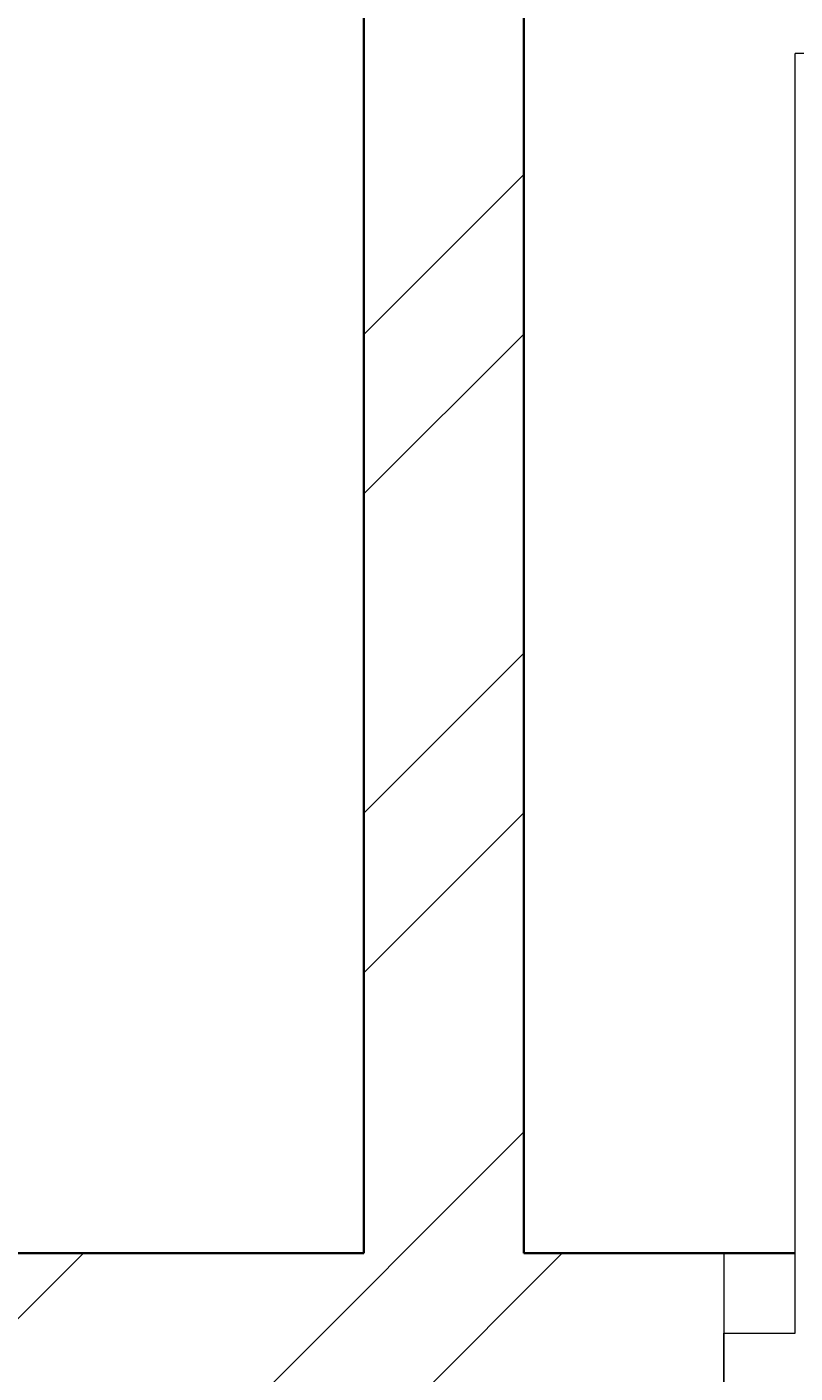
# Model space of a CAD drawing. Units: inches. Extents: x 1962 to 2771, y 1245 to 2660.
# Tile 53 of 114: x 2225 to 2247, y 2030 to 2068. Entities that reach past the tile are written whole.
import ezdxf

# ---------------------------------------------------------------- set-up
doc = ezdxf.new("R2010")
doc.units = ezdxf.units.IN
for name, color, linetype, lineweight in [('A-ANNO-DIMS', 2, 'Continuous', 18), ('A-DOOR', 3, 'Continuous', 18), ('A-WALL', 7, 'Continuous', 35), ('A-WALL-PATT', 252, 'Continuous', 13)]:
    doc.layers.add(name, color=color, linetype=linetype, lineweight=lineweight)
doc.styles.get("Standard").update_dxf_attribs({"font": 'arial.ttf'})
doc.dimstyles.get("Standard").update_dxf_attribs({"dimtxt": 0.18, "dimasz": 0.18, "dimexe": 0.18, "dimexo": 0.0625, "dimgap": 0.09, "dimtad": 0, "dimtih": 1, "dimtoh": 1, "dimdec": 4, "dimzin": 0, "dimdsep": 46, "dimtxsty": 'Standard', "dimcen": 0.09, "dimadec": 0, "dimazin": 0, "dimtfac": 1, "dimtdec": 4, "dimtofl": 0, "dimtmove": 0, "dimatfit": 3, "dimfxl": 1, "dimtolj": 1, "dimtzin": 0, "dimarcsym": 0})

# ---------------------------------------------------------------- blocks, each defined once
blk = doc.blocks.new('*D40')
at = {"layer": 'A-ANNO-DIMS', "color": 0, "lineweight": -2, "transparency": 16777216}
for p, q in [((2072.02, 2033.906), (2072.02, 2583.474)), ((2660.807, 2524.406), (2660.807, 2583.474)), ((2072.2, 2583.294), (2366.02, 2583.294)), ((2660.627, 2583.294), (2366.808, 2583.294))]:
    blk.add_line(p, q, dxfattribs=at)
at = {"layer": 'A-ANNO-DIMS', "color": 0, "transparency": 16777216}
for points in [[(2072.2, 2583.324), (2072.2, 2583.264), (2072.02, 2583.294)], [(2660.627, 2583.324), (2660.627, 2583.264), (2660.807, 2583.294)]]:
    blk.add_solid(points, dxfattribs=at)
at = {"layer": 'Defpoints', "color": 0, "transparency": 16777216}
for p in [(2660.807, 2583.294), (2660.807, 2524.344), (2072.02, 2033.844)]:
    blk.add_point(p, dxfattribs=at)
at = {"layer": 'A-ANNO-DIMS', "color": 0, "transparency": 16777216, "insert": (2366.414, 2583.294), "char_height": 0.18, "attachment_point": 5}
blk.add_mtext('\\A1;588.8', dxfattribs=at)

msp = doc.modelspace()

# ---------------------------------------------------------------- hatches: boundary and pattern name
at = {"layer": 'A-WALL-PATT'}
h = msp.add_hatch(dxfattribs=at)
h.set_pattern_fill('ANSI32', color=256)
h.paths.add_polyline_path([(2090.8074, 2467.3437), (2141.6481, 2467.3437), (2141.6481, 2469.5937), (2141.6481, 2471.8437), (2086.3074, 2471.8437), (2086.3074, 2422.5333), (2090.8074, 2422.5333)])
h.paths.add_polyline_path([(2282.7664, 2471.8437), (2204.8982, 2471.8437), (2204.8982, 2467.3437), (2234.8074, 2467.3437), (2234.8074, 2311.3437), (2228.7492, 2311.3437), (2228.7492, 2306.8437), (2234.8074, 2306.8437), (2331.9227, 2306.8437), (2331.9227, 2309.0937), (2331.9227, 2311.3437), (2239.3074, 2311.3437), (2239.3074, 2467.3437), (2282.7664, 2467.3437), (2282.7664, 2469.5937)])
h.paths.add_polyline_path([(2471.4531, 2519.8437), (2552.011, 2519.8437), (2564.3996, 2519.8437), (2564.3996, 2511.1389), (2568.8996, 2511.1389), (2568.8996, 2524.3437), (2466.9531, 2524.3437), (2466.9531, 2471.8437), (2450.0749, 2471.8437), (2446.4672, 2471.8437), (2446.4672, 2467.3437), (2450.0749, 2467.3437), (2475.9988, 2467.3437), (2475.9988, 2469.5937), (2475.9988, 2471.8437), (2471.4531, 2471.8437)])
h.paths.add_polyline_path([(2575.2231, 2469.5937), (2575.2231, 2471.8437), (2568.8996, 2471.8437), (2568.8996, 2487.1389), (2564.3996, 2487.1389), (2564.3996, 2471.8437), (2556.511, 2471.8437), (2499.2904, 2471.8437), (2499.2904, 2467.3437), (2507.8074, 2467.3437), (2507.8074, 2311.3437), (2414.863, 2311.3437), (2414.863, 2306.8437), (2512.3074, 2306.8437), (2517.0114, 2306.8437), (2517.0114, 2309.0937), (2517.0114, 2311.3437), (2512.3074, 2311.3437), (2512.3074, 2467.3437), (2575.2231, 2467.3437)])
h.paths.add_polyline_path([(2660.8074, 2471.8437), (2600.9602, 2471.8437), (2600.9602, 2467.3437), (2656.3074, 2467.3437), (2656.3074, 2432.5704), (2660.8074, 2432.5704)])
h.paths.add_polyline_path([(2660.8074, 2372.5704), (2656.3074, 2372.5704), (2656.3074, 2311.3437), (2600.276, 2311.3437), (2600.276, 2309.0937), (2600.276, 2306.8437), (2656.3074, 2306.8437), (2656.3074, 2296.2593), (2660.8074, 2296.2593)])
h.paths.add_polyline_path([(2572.3074, 2306.8437), (2577.1385, 2306.8437), (2577.1385, 2311.3437), (2551.082, 2311.3437), (2551.082, 2306.8437), (2567.8074, 2306.8437), (2567.8074, 2258.8437), (2540.0574, 2258.8437), (2540.0574, 2256.5937), (2540.0574, 2254.3437), (2567.8074, 2254.3437), (2656.3074, 2254.3437), (2656.3074, 2236.9085), (2660.8074, 2236.9085), (2660.8074, 2272.2593), (2656.3074, 2272.2593), (2656.3074, 2258.8437), (2572.3074, 2258.8437)])
h.paths.add_polyline_path([(2512.3074, 2254.3437), (2518.8716, 2254.3437), (2518.8716, 2256.5937), (2518.8716, 2258.8437), (2507.8074, 2258.8437), (2507.8074, 2177.8437), (2567.8074, 2177.8437), (2567.8074, 2172.9628), (2572.3074, 2172.9628), (2572.3074, 2177.8437), (2656.3074, 2177.8437), (2656.3074, 2166.4846), (2660.8074, 2166.4846), (2660.8074, 2200.9085), (2656.3074, 2200.9085), (2656.3074, 2182.3437), (2512.3074, 2182.3437)])
h.paths.add_polyline_path([(2656.3074, 2129.8437), (2572.3074, 2129.8437), (2572.3074, 2150.3044), (2570.0574, 2150.3044), (2567.8074, 2150.3044), (2567.8074, 2129.8437), (2507.8074, 2129.8437), (2507.8074, 2116.3027), (2510.0574, 2116.3027), (2512.3074, 2116.3027), (2512.3074, 2125.3437), (2567.8074, 2125.3437), (2572.3074, 2125.3437), (2656.3074, 2125.3437)])
h.paths.add_polyline_path([(2090.8074, 2362.5333), (2086.3074, 2362.5333), (2086.3074, 2298.6242), (2090.8074, 2298.6242), (2090.8074, 2306.8437), (2174.8074, 2306.8437), (2174.8074, 2286.4178), (2179.3074, 2286.4178), (2179.3074, 2306.8437), (2192.8641, 2306.8437), (2192.8641, 2309.0937), (2192.8641, 2311.3437), (2090.8074, 2311.3437)])
h.paths.add_polyline_path([(2209.156, 2258.8437), (2179.3074, 2258.8437), (2179.3074, 2263.2236), (2177.0574, 2263.2236), (2174.8074, 2263.2236), (2174.8074, 2258.8437), (2090.8074, 2258.8437), (2090.8074, 2274.6242), (2086.3074, 2274.6242), (2086.3074, 2238.2967), (2088.5574, 2238.2967), (2090.8074, 2238.2967), (2090.8074, 2254.3437), (2209.156, 2254.3437)])
h.paths.add_polyline_path([(2090.8074, 2177.8437), (2234.8074, 2177.8437), (2234.8074, 2173.1428), (2239.3074, 2173.1428), (2239.3074, 2258.8437), (2230.8442, 2258.8437), (2230.8442, 2256.5937), (2230.8442, 2254.3437), (2234.8074, 2254.3437), (2234.8074, 2182.3437), (2090.8074, 2182.3437), (2090.8074, 2202.2967), (2086.3074, 2202.2967), (2086.3074, 2140.0389), (2090.8074, 2140.0389)])
h.paths.add_polyline_path([(2090.8074, 2080.0389), (2086.3074, 2080.0389), (2086.3074, 2033.8437), (2090.8074, 2033.8437)], flags=17)
h.paths.add_polyline_path([(2244.9405, 2033.8437), (2239.3074, 2033.8437), (2239.3074, 2142.0665), (2237.2592, 2142.0665), (2234.8074, 2142.0665), (2234.8074, 2033.8437), (2090.8074, 2033.8437), (2076.5204, 2033.8437), (2072.0204, 2033.8437), (2072.0204, 2000.4493), (2076.5204, 2000.4493), (2076.5204, 2029.3437), (2090.8074, 2029.3437), (2244.9405, 2029.3437), (2244.9405, 2031.5937)])
h.paths.add_polyline_path([(2234.8074, 1933.3437), (2076.5204, 1933.3437), (2076.5204, 1952.4493), (2074.2704, 1952.4493), (2072.0204, 1952.4493), (2072.0204, 1933.3437), (2072.0204, 1928.8437), (2234.8074, 1928.8437)])
h.paths.add_polyline_path([(2090.8074, 1928.8437), (2086.3074, 1928.8437), (2086.3074, 1906.5013), (2090.8074, 1906.5013)])
h.paths.add_polyline_path([(2090.8074, 1846.5013), (2086.3074, 1846.5013), (2086.3074, 1769.9917), (2088.5574, 1769.9917), (2090.8074, 1769.9917), (2090.8074, 1780.3437), (2234.8074, 1780.3437), (2234.8074, 1708.3437), (2230.3764, 1708.3437), (2230.3764, 1703.8437), (2239.3074, 1703.8437), (2239.3074, 1792.6669), (2237.0574, 1792.6669), (2234.8074, 1792.6669), (2234.8074, 1784.8437), (2090.8074, 1784.8437)])
h.paths.add_polyline_path([(2239.3074, 1928.8437), (2244.9405, 1928.8437), (2244.9405, 1931.0937), (2244.9405, 1933.3437), (2234.8074, 1933.3437), (2234.8074, 1928.8437), (2234.8074, 1825.5949), (2239.3074, 1825.5949)])
h.paths.add_polyline_path([(2148.0425, 1649.0937), (2148.0425, 1651.3437), (2090.8074, 1651.3437), (2090.8074, 1646.8437), (2148.0425, 1646.8437)], flags=0)
h.paths.add_polyline_path([(2207.5601, 1708.3437), (2090.8074, 1708.3437), (2090.8074, 1703.8437), (2174.8074, 1703.8437), (2174.8074, 1651.3437), (2170.4457, 1651.3437), (2170.4457, 1646.8437), (2195.9924, 1646.8437), (2195.9924, 1649.0937), (2195.9924, 1651.3437), (2179.3074, 1651.3437), (2179.3074, 1703.8437), (2207.5601, 1703.8437), (2207.5601, 1706.0937)])
h.paths.add_polyline_path([(2090.8074, 1733.9917), (2086.3074, 1733.9917), (2086.3074, 1696.1032), (2088.5574, 1696.1032), (2090.8074, 1696.1032)])
h.paths.add_polyline_path([(2090.8074, 1672.1032), (2086.3074, 1672.1032), (2086.3074, 1600.3335), (2090.8074, 1600.3335)])
h.paths.add_polyline_path([(2090.8074, 1540.3335), (2086.3074, 1540.3335), (2086.3074, 1486.3437), (2139.6766, 1486.3437), (2139.6766, 1490.8437), (2090.8074, 1490.8437)])
h.paths.add_polyline_path([(2302.3876, 1490.8437), (2239.3074, 1490.8437), (2239.3074, 1646.8437), (2335.9994, 1646.8437), (2335.9994, 1651.3437), (2229.884, 1651.3437), (2229.884, 1646.8437), (2234.8074, 1646.8437), (2234.8074, 1490.8437), (2202.7103, 1490.8437), (2202.7103, 1488.5937), (2202.7103, 1486.3437), (2275.0699, 1486.3437), (2275.0699, 1475.772), (2279.5699, 1475.772), (2279.5699, 1486.3437), (2302.3876, 1486.3437)])
h.paths.add_polyline_path([(2279.5699, 1451.772), (2275.0699, 1451.772), (2275.0699, 1438.3437), (2174.8074, 1438.3437), (2174.8074, 1486.3437), (2179.7922, 1486.3437), (2179.7922, 1490.8437), (2163.3585, 1490.8437), (2163.3585, 1488.5937), (2163.3585, 1486.3437), (2170.3074, 1486.3437), (2170.3074, 1433.8437), (2279.5699, 1433.8437)])
h.paths.add_polyline_path([(2427.2363, 1490.8437), (2375.8074, 1490.8437), (2375.8074, 1646.8437), (2381.6401, 1646.8437), (2381.6401, 1651.3437), (2365.887, 1651.3437), (2365.887, 1649.0937), (2365.887, 1646.8437), (2371.3074, 1646.8437), (2371.3074, 1490.8437), (2327.5627, 1490.8437), (2327.5627, 1488.5937), (2327.5627, 1486.3437), (2371.3074, 1486.3437), (2371.3074, 1433.8437), (2375.8074, 1433.8437), (2375.8074, 1486.3437), (2427.2363, 1486.3437)])
h.paths.add_polyline_path([(2512.3074, 1646.8437), (2519.4351, 1646.8437), (2519.4351, 1649.0937), (2519.4351, 1651.3437), (2507.8074, 1651.3437), (2416.0063, 1651.3437), (2416.0063, 1649.0937), (2416.0063, 1646.8437), (2507.8074, 1646.8437), (2507.8074, 1490.8437), (2497.0532, 1490.8437), (2497.0532, 1488.5937), (2497.0532, 1486.3437), (2574.9344, 1486.3437), (2574.9344, 1476.0181), (2579.4344, 1476.0181), (2579.4344, 1486.3437), (2584.4872, 1486.3437), (2584.3074, 1490.8437), (2512.3074, 1490.8437)])
h.paths.add_polyline_path([(2470.5091, 1486.3437), (2473.9767, 1486.3437), (2473.9767, 1490.8437), (2449.6605, 1490.8437), (2449.6605, 1488.5937), (2449.6605, 1486.3437), (2466.0091, 1486.3437), (2466.0091, 1433.8437), (2470.5091, 1433.8437), (2579.4344, 1433.8437), (2579.4344, 1452.0181), (2574.9344, 1452.0181), (2574.9344, 1438.3437), (2554.5091, 1438.3437), (2470.5091, 1438.3437)])
h.paths.add_polyline_path([(2656.3074, 1490.8437), (2611.86, 1490.8437), (2611.86, 1486.3437), (2656.3074, 1486.3437)])
h.paths.add_polyline_path([(2660.8074, 1532.7007), (2658.5574, 1532.7007), (2656.3074, 1532.7007), (2656.3074, 1486.3437), (2660.8074, 1486.3437)])
h.paths.add_polyline_path([(2660.8074, 1664.9663), (2656.3074, 1664.9663), (2656.3074, 1651.3437), (2602.2313, 1651.3437), (2602.2313, 1646.8437), (2656.3074, 1646.8437), (2656.3074, 1592.7007), (2660.8074, 1592.7007)])
h.paths.add_polyline_path([(2660.8074, 1724.5221), (2656.3074, 1724.5221), (2656.3074, 1703.8437), (2542.4725, 1703.8437), (2542.4725, 1699.3437), (2567.8074, 1699.3437), (2567.8074, 1651.3437), (2552.7766, 1651.3437), (2552.7766, 1649.0937), (2552.7766, 1646.8437), (2577.2878, 1646.8437), (2577.2878, 1649.0937), (2577.2878, 1651.3437), (2572.3074, 1651.3437), (2572.3074, 1699.3437), (2656.3074, 1699.3437), (2656.3074, 1688.9663), (2660.8074, 1688.9663)])
h.paths.add_polyline_path([(2660.8074, 1880.6524), (2656.3074, 1880.6524), (2656.3074, 1832.8437), (2512.3074, 1832.8437), (2512.3074, 1837.8959), (2507.8074, 1837.8959), (2507.8074, 1828.3437), (2567.8074, 1828.3437), (2567.8074, 1804.3437), (2572.3074, 1804.3437), (2572.3074, 1828.3437), (2656.3074, 1828.3437), (2656.3074, 1818.6778), (2660.8074, 1818.6778)])
h.paths.add_polyline_path([(2660.8074, 1794.6778), (2656.3074, 1794.6778), (2656.3074, 1780.3437), (2572.3074, 1780.3437), (2572.3074, 1783.0303), (2570.0574, 1783.0303), (2567.8074, 1783.0303), (2567.8074, 1780.3437), (2507.8074, 1780.3437), (2507.8074, 1699.3437), (2517.8858, 1699.3437), (2517.8858, 1701.5937), (2517.8858, 1703.8437), (2512.3074, 1703.8437), (2512.3074, 1775.8437), (2656.3074, 1775.8437), (2656.3074, 1760.5221), (2660.8074, 1760.5221)])
h.paths.add_polyline_path([(2660.8074, 1981.3437), (2660.8074, 2020.2808), (2658.5574, 2020.2808), (2656.3074, 2020.2808), (2656.3074, 1981.3437), (2512.3074, 1981.3437), (2512.3074, 2086.6996), (2507.8074, 2086.6996), (2507.8074, 1981.3437), (2375.8074, 1981.3437), (2375.8074, 1986.8505), (2373.5574, 1986.8505), (2371.3074, 1986.8505), (2371.3074, 1973.2607), (2375.8074, 1973.2607), (2375.8074, 1976.8437), (2507.8074, 1976.8437), (2507.8074, 1865.4281), (2510.0574, 1865.4281), (2512.3074, 1865.4281), (2512.3074, 1976.8437), (2660.8074, 1976.8437)])
h.paths.add_polyline_path([(2375.8074, 1940.297), (2373.5574, 1940.297), (2371.3074, 1940.297), (2371.3074, 1933.3437), (2278.4434, 1933.3437), (2278.4434, 1928.8437), (2371.3074, 1928.8437), (2371.3074, 1651.3437), (2375.8074, 1651.3437)])
h.paths.add_polyline_path([(2660.8074, 1976.8437), (2656.3074, 1976.8437), (2656.3074, 1940.6524), (2660.8074, 1940.6524)], flags=17)
h.paths.add_polyline_path([(2660.8074, 2142.4846), (2656.3074, 2142.4846), (2656.3074, 2080.2808), (2660.8074, 2080.2808)])
h.paths.add_polyline_path([(2381.4189, 2311.3437), (2375.8074, 2311.3437), (2375.8074, 2467.3437), (2424.7242, 2467.3437), (2424.7242, 2469.5937), (2424.7242, 2471.8437), (2375.8074, 2471.8437), (2375.8074, 2524.3437), (2371.3074, 2524.3437), (2371.3074, 2471.8437), (2307.2097, 2471.8437), (2307.2097, 2467.3437), (2371.3074, 2467.3437), (2371.3074, 2311.3437), (2366.8901, 2311.3437), (2366.8901, 2306.8437), (2371.3074, 2306.8437), (2371.3074, 2033.8437), (2279.6589, 2033.8437), (2279.6589, 2029.3437), (2371.3074, 2029.3437), (2371.3074, 2014.2598), (2375.8074, 2014.2598), (2375.8074, 2306.8437), (2381.4189, 2306.8437)])
h.paths.add_polyline_path([(2263.3074, 2524.3437), (2170.3074, 2524.3437), (2170.3074, 2519.8437), (2170.3074, 2471.8437), (2165.0312, 2471.8437), (2165.0312, 2467.3437), (2179.6721, 2467.3437), (2179.6721, 2469.5161), (2179.6721, 2471.8437), (2174.8074, 2471.8437), (2174.8074, 2519.8437), (2258.8074, 2519.8437), (2258.8074, 2511.6436), (2263.3074, 2511.6436)])
h.paths.add_polyline_path([(2245.0232, 1361.4123), (2492.9468, 1361.4123), (2492.9468, 1398.505), (2245.0232, 1398.505)], flags=9)
h.paths.add_polyline_path([(2388.1434, 2086.6936), (2425.0704, 2086.6936), (2425.0704, 2105.3509), (2388.1434, 2105.3509)], flags=9)
h.paths.add_polyline_path([(2404.922, 2242.6744), (2445.7337, 2242.6744), (2445.7337, 2261.3318), (2404.922, 2261.3318)], flags=9)
h.paths.add_polyline_path([(2269.4107, 2156.7935), (2306.3378, 2156.7935), (2306.3378, 2175.4508), (2269.4107, 2175.4508)], flags=9)
h.paths.add_polyline_path([(2269.3277, 2233.4343), (2306.2547, 2233.4343), (2306.2547, 2252.0917), (2269.3277, 2252.0917)], flags=9)
h.paths.add_polyline_path([(2431.6052, 2320.6922), (2470.4456, 2320.6922), (2470.4456, 2339.3495), (2431.6052, 2339.3495)], flags=25)
h.paths.add_polyline_path([(2249.6902, 2315.7608), (2288.5306, 2315.7608), (2288.5306, 2334.4182), (2249.6902, 2334.4182)], flags=25)
h.paths.add_polyline_path([(2096.9301, 2314.3181), (2135.7704, 2314.3181), (2135.7704, 2332.9755), (2096.9301, 2332.9755)], flags=25)
h.paths.add_polyline_path([(2134.3475, 2285.7089), (2161.4655, 2285.7089), (2161.4655, 2304.3662), (2134.3475, 2304.3662)], flags=9)
h.paths.add_polyline_path([(2126.5155, 2209.4076), (2159.9227, 2209.4076), (2159.9227, 2228.065), (2126.5155, 2228.065)], flags=25)
h.paths.add_polyline_path([(2110.5753, 2141.5299), (2149.4157, 2141.5299), (2149.4157, 2160.1872), (2110.5753, 2160.1872)], flags=25)
h.paths.add_polyline_path([(2249.8618, 1968.3317), (2286.3966, 1968.3317), (2286.3966, 1986.989), (2249.8618, 1986.989)], flags=9)
h.paths.add_polyline_path([(2395.9507, 1777.0051), (2436.7624, 1777.0051), (2436.7624, 1795.6625), (2395.9507, 1795.6625)], flags=9)
h.paths.add_polyline_path([(2398.5259, 1888.5651), (2435.0062, 1888.5651), (2435.0062, 1907.2224), (2398.5259, 1907.2224)], flags=25)
h.paths.add_polyline_path([(2259.3506, 1728.3559), (2296.2776, 1728.3559), (2296.2776, 1747.0132), (2259.3506, 1747.0132)], flags=9)
h.paths.add_polyline_path([(2271.3698, 1845.268), (2308.2968, 1845.268), (2308.2968, 1863.9253), (2271.3698, 1863.9253)], flags=9)
h.paths.add_polyline_path([(2120.9355, 1786.3027), (2159.7759, 1786.3027), (2159.7759, 1804.9601), (2120.9355, 1804.9601)], flags=25)
h.paths.add_polyline_path([(2121.3164, 1732.1043), (2154.7236, 1732.1043), (2154.7236, 1750.7616), (2121.3164, 1750.7616)], flags=25)
h.paths.add_polyline_path([(2118.3706, 1678.8997), (2147.5282, 1678.8997), (2147.5282, 1697.557), (2118.3706, 1697.557)], flags=25)
h.paths.add_polyline_path([(2385.9227, 1493.557), (2424.763, 1493.557), (2424.763, 1512.2143), (2385.9227, 1512.2143)], flags=25)
h.paths.add_polyline_path([(2248.7058, 1500.0256), (2287.5462, 1500.0256), (2287.5462, 1518.6829), (2248.7058, 1518.6829)], flags=25)
h.paths.add_polyline_path([(2104.1669, 1617.3771), (2143.0073, 1617.3771), (2143.0073, 1636.0344), (2104.1669, 1636.0344)], flags=9)
h.paths.add_polyline_path([(2096.0714, 1447.8824), (2137.3845, 1447.8824), (2137.3845, 1458.1859), (2096.0714, 1458.1859)], flags=9)
h.paths.add_polyline_path([(2180.6114, 1440.325), (2209.7689, 1440.325), (2209.7689, 1458.9823), (2180.6114, 1458.9823)], flags=25)
h.paths.add_polyline_path([(2316.1698, 1447.9637), (2357.4829, 1447.9637), (2357.4829, 1458.2673), (2316.1698, 1458.2673)], flags=9)
h.paths.add_polyline_path([(2397.6187, 1447.9637), (2438.9318, 1447.9637), (2438.9318, 1458.2673), (2397.6187, 1458.2673)], flags=9)
h.paths.add_polyline_path([(2473.0778, 1439.5953), (2502.2354, 1439.5953), (2502.2354, 1458.2527), (2473.0778, 1458.2527)], flags=25)
h.paths.add_polyline_path([(2589.7027, 1447.8819), (2631.0158, 1447.8819), (2631.0158, 1458.1855), (2589.7027, 1458.1855)], flags=9)
h.paths.add_polyline_path([(2522.4009, 1497.5285), (2561.2413, 1497.5285), (2561.2413, 1516.1859), (2522.4009, 1516.1859)], flags=25)
h.paths.add_polyline_path([(2579.6565, 1671.3482), (2608.8141, 1671.3482), (2608.8141, 1690.0056), (2579.6565, 1690.0056)], flags=25)
h.paths.add_polyline_path([(2544.7038, 1725.5064), (2578.1111, 1725.5064), (2578.1111, 1744.1637), (2544.7038, 1744.1637)], flags=25)
h.paths.add_polyline_path([(2578.1191, 1807.472), (2607.2766, 1807.472), (2607.2766, 1826.1293), (2578.1191, 1826.1293)], flags=25)
h.paths.add_polyline_path([(2595.0614, 1835.1839), (2633.9018, 1835.1839), (2633.9018, 1853.8413), (2595.0614, 1853.8413)], flags=25)
h.paths.add_polyline_path([(2567.0097, 2097.7035), (2605.8501, 2097.7035), (2605.8501, 2116.3609), (2567.0097, 2116.3609)], flags=9)
h.paths.add_polyline_path([(2586.644, 2134.6454), (2615.8015, 2134.6454), (2615.8015, 2153.3027), (2586.644, 2153.3027)], flags=9)
h.paths.add_polyline_path([(2544.6185, 2212.6783), (2578.0258, 2212.6783), (2578.0258, 2231.3356), (2544.6185, 2231.3356)], flags=25)
h.paths.add_polyline_path([(2577.0273, 2256.9023), (2606.1849, 2256.9023), (2606.1849, 2275.5597), (2577.0273, 2275.5597)], flags=24)
h.paths.add_polyline_path([(2605.2683, 2315.2821), (2644.1087, 2315.2821), (2644.1087, 2333.9395), (2605.2683, 2333.9395)], flags=25)
h.paths.add_polyline_path([(2583.1244, 2496.1815), (2624.4375, 2496.1815), (2624.4375, 2506.4851), (2583.1244, 2506.4851)], flags=9)
h.paths.add_polyline_path([(2474.761, 2497.0823), (2503.9185, 2497.0823), (2503.9185, 2515.7397), (2474.761, 2515.7397)], flags=25)
h.paths.add_polyline_path([(2387.5787, 2494.2563), (2428.902, 2494.2563), (2428.902, 2504.5598), (2387.5787, 2504.5598)], flags=9)
h.paths.add_polyline_path([(2300.1657, 2500.1564), (2341.4788, 2500.1564), (2341.4788, 2510.46), (2300.1657, 2510.46)], flags=25)
h.paths.add_polyline_path([(2176.8589, 2497.5843), (2206.0165, 2497.5843), (2206.0165, 2516.2416), (2176.8589, 2516.2416)], flags=25)
h.paths.add_polyline_path([(2097.4668, 2494.9762), (2138.7799, 2494.9762), (2138.7799, 2505.2798), (2097.4668, 2505.2798)], flags=9)

# ---------------------------------------------------------------- linework, layer by layer
at = {"layer": 'A-DOOR'}
for p, q in [((2246.9405, 2031.5937), (2246.9405, 2067.5937)), ((2244.9405, 2033.8437), (2244.9405, 2029.3437)), ((2244.9405, 2029.3437), (2244.9405, 2031.5937)), ((2244.9405, 2031.5937), (2246.9405, 2031.5937))]:
    msp.add_line(p, q, dxfattribs=at)
msp.add_arc((2246.9405, 2036.4879), 31.1058, 350.94752, 90, dxfattribs=at)
at = {"layer": 'A-WALL'}
for p, q in [((2234.8074, 2143.4621), (2234.8074, 2033.8437)), ((2239.3074, 2142.0665), (2239.3074, 2033.8437)), ((2090.8074, 2033.8437), (2234.8074, 2033.8437)), ((2239.3074, 2033.8437), (2246.9405, 2033.8437))]:
    msp.add_line(p, q, dxfattribs=at)

# ---------------------------------------------------------------- dimensions: what is measured, and where the dimension line sits
at = {"layer": 'A-ANNO-DIMS'}
dim = msp.add_linear_dim(base=(2660.8074, 2583.2937), p1=(2072.0204, 2033.8437), p2=(2660.8074, 2524.3437), dimstyle='Standard', override={"dimdec": 1, "dimlfac": 1, "dimrnd": 0, "dimzin": 0, "dimdsep": 46, "dimlunit": 2}, dxfattribs=at)
dim.commit()
dim.dimension.update_dxf_attribs({"geometry": '*D40', "text_midpoint": (2366.4139, 2583.2937)})

doc.saveas('drawing.dxf')
